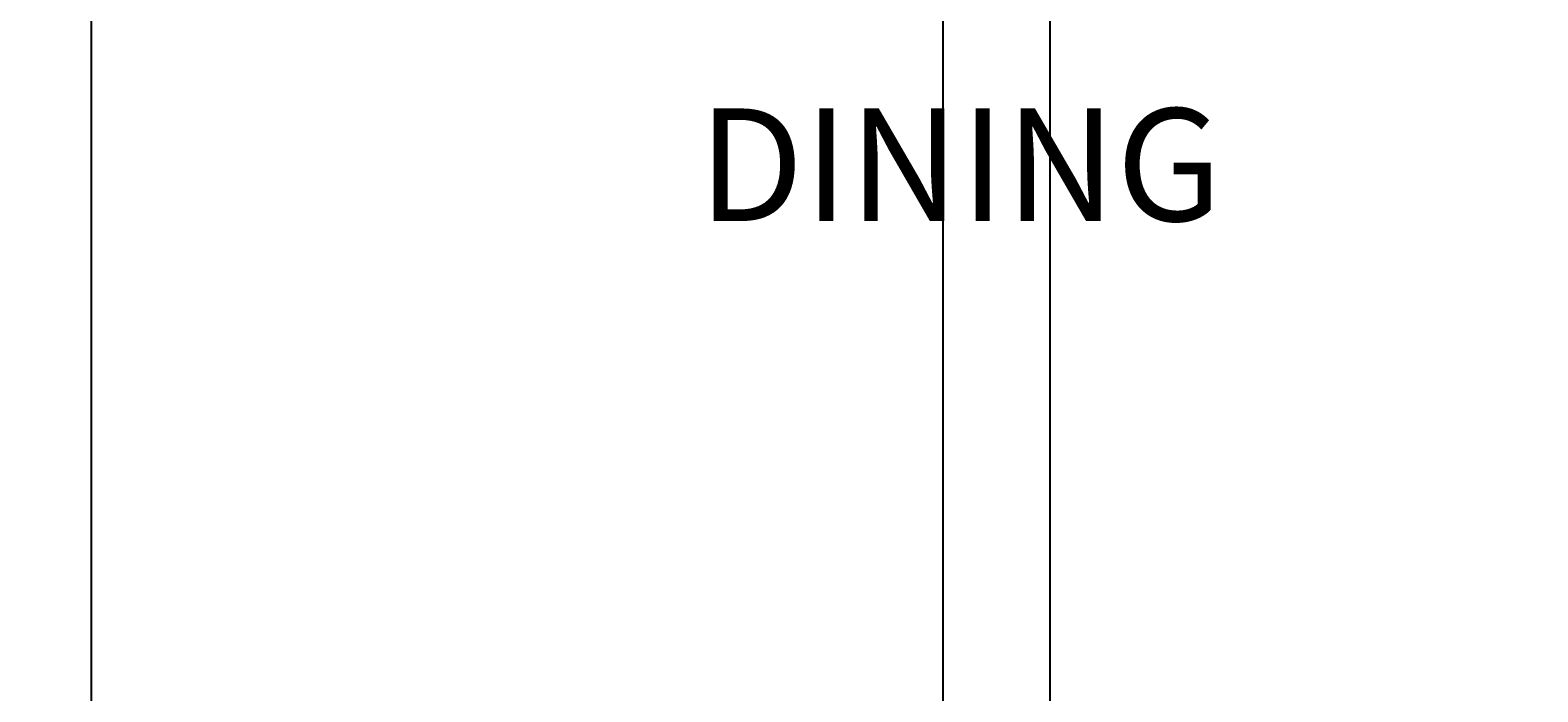
# Model space of a CAD drawing. Units: inches. Extents: x 2549 to 3108, y 1683 to 2362.
# Tile 7 of 30: x 2678 to 2762, y 1979 to 2016. Entities that reach past the tile are written whole.
import ezdxf

# ---------------------------------------------------------------- set-up
doc = ezdxf.new("R2010")
doc.units = ezdxf.units.IN
for name, color, linetype, lineweight in [('A-ANNO-DIMS', 2, 'Continuous', 18), ('A-AREA-IDEN', 7, 'Continuous', 18), ('A-FURN-PATT', 9, 'Continuous', 13)]:
    doc.layers.add(name, color=color, linetype=linetype, lineweight=lineweight)
doc.layers.add('C-PKNG-VEHI-PATT', color=251, linetype='Continuous', lineweight=13, true_color=0x636466)
doc.layers.add('C-PVMT-PATT', color=9, linetype='Continuous', lineweight=13, true_color=0xc7c8ca)
doc.styles.get("Standard").update_dxf_attribs({"font": 'arial.ttf'})
doc.dimstyles.get("Standard").update_dxf_attribs({"dimtxt": 0.18, "dimasz": 0.18, "dimexe": 0.18, "dimexo": 0.0625, "dimgap": 0.09, "dimtad": 0, "dimtih": 1, "dimtoh": 1, "dimdec": 4, "dimzin": 0, "dimdsep": 46, "dimtxsty": 'Standard', "dimcen": 0.09, "dimadec": 0, "dimazin": 0, "dimtfac": 1, "dimtdec": 4, "dimtofl": 0, "dimtmove": 0, "dimatfit": 3, "dimfxl": 1, "dimtolj": 1, "dimtzin": 0, "dimarcsym": 0})

# ---------------------------------------------------------------- blocks, each defined once
blk = doc.blocks.new('*D42')
at = {"layer": 'A-ANNO-DIMS', "color": 0, "lineweight": -2, "transparency": 16777216}
for p, q in [((2638.643, 2080.461), (2638.643, 1683.444)), ((2728.643, 2080.461), (2728.643, 1683.444)), ((2638.823, 1683.624), (2683.424, 1683.624)), ((2728.463, 1683.624), (2683.861, 1683.624))]:
    blk.add_line(p, q, dxfattribs=at)
at = {"layer": 'A-ANNO-DIMS', "color": 0, "transparency": 16777216}
for points in [[(2638.823, 1683.654), (2638.823, 1683.594), (2638.643, 1683.624)], [(2728.463, 1683.654), (2728.463, 1683.594), (2728.643, 1683.624)]]:
    blk.add_solid(points, dxfattribs=at)
at = {"layer": 'Defpoints', "color": 0, "transparency": 16777216}
for p in [(2638.643, 2080.524), (2728.643, 2080.524), (2728.643, 1683.624)]:
    blk.add_point(p, dxfattribs=at)
at = {"layer": 'A-ANNO-DIMS', "color": 0, "transparency": 16777216, "insert": (2683.643, 1683.624), "char_height": 0.18, "attachment_point": 5}
blk.add_mtext('\\A1;90', dxfattribs=at)
blk = doc.blocks.new('*D43')
at = {"layer": 'A-ANNO-DIMS', "color": 0, "lineweight": -2, "transparency": 16777216}
for p, q in [((2734.643, 2080.461), (2734.643, 1683.444)), ((2806.643, 2080.461), (2806.643, 1683.444)), ((2734.823, 1683.624), (2770.425, 1683.624)), ((2806.463, 1683.624), (2770.86, 1683.624))]:
    blk.add_line(p, q, dxfattribs=at)
at = {"layer": 'A-ANNO-DIMS', "color": 0, "transparency": 16777216}
for points in [[(2734.823, 1683.654), (2734.823, 1683.594), (2734.643, 1683.624)], [(2806.463, 1683.654), (2806.463, 1683.594), (2806.643, 1683.624)]]:
    blk.add_solid(points, dxfattribs=at)
at = {"layer": 'Defpoints', "color": 0, "transparency": 16777216}
for p in [(2734.643, 2080.524), (2806.643, 2080.524), (2806.643, 1683.624)]:
    blk.add_point(p, dxfattribs=at)
at = {"layer": 'A-ANNO-DIMS', "color": 0, "transparency": 16777216, "insert": (2770.643, 1683.624), "char_height": 0.18, "attachment_point": 5}
blk.add_mtext('\\A1;72', dxfattribs=at)
blk = doc.blocks.new('*D44')
at = {"layer": 'A-ANNO-DIMS', "color": 0, "lineweight": -2, "transparency": 16777216}
for p, q in [((2662.643, 2040.993), (2662.643, 1683.444)), ((2806.643, 2016.129), (2806.643, 1683.444)), ((2662.823, 1683.624), (2734.363, 1683.624)), ((2806.463, 1683.624), (2734.923, 1683.624))]:
    blk.add_line(p, q, dxfattribs=at)
at = {"layer": 'A-ANNO-DIMS', "color": 0, "transparency": 16777216}
for points in [[(2662.823, 1683.654), (2662.823, 1683.594), (2662.643, 1683.624)], [(2806.463, 1683.654), (2806.463, 1683.594), (2806.643, 1683.624)]]:
    blk.add_solid(points, dxfattribs=at)
at = {"layer": 'Defpoints', "color": 0, "transparency": 16777216}
for p in [(2662.643, 2041.056), (2806.643, 2016.191), (2806.643, 1683.624)]:
    blk.add_point(p, dxfattribs=at)
at = {"layer": 'A-ANNO-DIMS', "color": 0, "transparency": 16777216, "insert": (2734.643, 1683.624), "char_height": 0.18, "attachment_point": 5}
blk.add_mtext('\\A1;144', dxfattribs=at)
blk = doc.blocks.new('*D59')
at = {"layer": 'A-ANNO-DIMS', "color": 0, "lineweight": -2, "transparency": 16777216}
for p, q in [((2680.978, 1761.586), (2680.978, 2362.323)), ((2786.158, 1761.586), (2786.158, 2362.323)), ((2681.158, 2362.143), (2733.112, 2362.143)), ((2785.978, 2362.143), (2734.023, 2362.143))]:
    blk.add_line(p, q, dxfattribs=at)
at = {"layer": 'A-ANNO-DIMS', "color": 0, "transparency": 16777216}
for points in [[(2681.158, 2362.173), (2681.158, 2362.113), (2680.978, 2362.143)], [(2785.978, 2362.173), (2785.978, 2362.113), (2786.158, 2362.143)]]:
    blk.add_solid(points, dxfattribs=at)
at = {"layer": 'Defpoints', "color": 0, "transparency": 16777216}
for p in [(2786.158, 2362.143), (2680.978, 1761.524), (2786.158, 1761.524)]:
    blk.add_point(p, dxfattribs=at)
at = {"layer": 'A-ANNO-DIMS', "color": 0, "transparency": 16777216, "insert": (2733.568, 2362.143), "char_height": 0.18, "attachment_point": 5}
blk.add_mtext('\\A1;105.18', dxfattribs=at)

msp = doc.modelspace()

# ---------------------------------------------------------------- hatches: boundary and pattern name
at = {"layer": 'A-FURN-PATT', "transparency": 33554567}
h = msp.add_hatch(color=256, dxfattribs=at)
h.dxf.hatch_style = 1
h.paths.add_polyline_path([(2708.7147, 2271.6737), (2675.2813, 2271.6737), (2675.2813, 2262.0404), (2708.7147, 2262.0404)])
h.paths.add_polyline_path([(2980.8246, 2271.6737), (2947.3913, 2271.6737), (2947.3913, 2262.0404), (2980.8246, 2262.0404)])
h.paths.add_polyline_path([(2748.8496, 2101.6383), (2798.148, 2101.6383), (2798.148, 2111.4248), (2748.8496, 2111.4248)], flags=9)
h.paths.add_polyline_path([(2685.2081, 2101.489), (2719.3253, 2101.489), (2719.3253, 2111.2819), (2685.2081, 2111.2819)], flags=9)
h.paths.add_polyline_path([(2814.6852, 1907.1328), (2847.8384, 1907.1328), (2847.8384, 1916.9258), (2814.6852, 1916.9258)], flags=9)
h.paths.add_polyline_path([(2814.3906, 1835.5864), (2848.0172, 1835.5864), (2848.0172, 1845.3794), (2814.3906, 1845.3794)], flags=9)
h.paths.add_polyline_path([(2800.5245, 1759.1674), (2853.7435, 1759.1674), (2853.7435, 1768.954), (2800.5245, 1768.954)], flags=9)
h.paths.add_polyline_path([(2972.4611, 1807.3305), (3015.3943, 1807.3305), (3015.3943, 1817.117), (2972.4611, 1817.117)], flags=9)
h.paths.add_polyline_path([(2902.3327, 1888.6731), (2937.9131, 1888.6731), (2937.9131, 1898.4661), (2902.3327, 1898.4661)], flags=9)
h.paths.add_polyline_path([(2712.1779, 1878.9039), (2754.1257, 1878.9039), (2754.1257, 1888.6904), (2712.1779, 1888.6904)], flags=9)
h.paths.add_polyline_path([(2614.0056, 2012.812), (2650.0251, 2012.812), (2650.0251, 2022.4371), (2614.0056, 2022.4371)], flags=9)
h.paths.add_polyline_path([(2713.3129, 2003.1645), (2747.4237, 2003.1645), (2747.4237, 2012.951), (2713.3129, 2012.951)], flags=9)
h.paths.add_polyline_path([(2950.1379, 2001.6934), (2982.2992, 2001.6934), (2982.2992, 2011.48), (2950.1379, 2011.48)], flags=9)
h.paths.add_polyline_path([(2940.864, 2238.5537), (2997.5066, 2238.5537), (2997.5066, 2248.3466), (2940.864, 2248.3466)], flags=9)
h.paths.add_polyline_path([(2821.5457, 2202.8348), (2855.663, 2202.8348), (2855.663, 2212.6278), (2821.5457, 2212.6278)], flags=9)
h.paths.add_polyline_path([(2661.8026, 2238.6249), (2718.4451, 2238.6249), (2718.4451, 2248.4179), (2661.8026, 2248.4179)], flags=9)
h = msp.add_hatch(color=256, dxfattribs=at)
h.dxf.hatch_style = 1
h.paths.add_polyline_path([(2906.5064, 1905.2148), (2905.2584, 1904.3827), (2907.0611, 1900.7772), (2908.3092, 1901.6092)])
h.paths.add_polyline_path([(2936.522, 1914.8044), (2935.2739, 1915.6364), (2932.6391, 1912.5856), (2933.8871, 1911.7535)])
h.paths.add_polyline_path([(2950.2508, 1905.6518), (2949.0027, 1906.4839), (2947.1999, 1902.8783), (2948.448, 1902.0463)])
h.paths.add_polyline_path([(2958.5713, 1918.1326), (2956.9072, 1919.242), (2952.4696, 1908.98, 1.3874274), (2954.9657, 1907.3159)])
h.paths.add_polyline_path([(2945.2585, 1927.0078), (2943.5944, 1928.1172), (2934.9965, 1920.6287, 1.3874274), (2937.4927, 1918.9646)])
h.paths.add_polyline_path([(2748.8496, 2101.6383), (2798.148, 2101.6383), (2798.148, 2111.4248), (2748.8496, 2111.4248)], flags=9)
h.paths.add_polyline_path([(2685.2081, 2101.489), (2719.3253, 2101.489), (2719.3253, 2111.2819), (2685.2081, 2111.2819)], flags=9)
h.paths.add_polyline_path([(2814.6852, 1907.1328), (2847.8384, 1907.1328), (2847.8384, 1916.9258), (2814.6852, 1916.9258)], flags=9)
h.paths.add_polyline_path([(2814.3906, 1835.5864), (2848.0172, 1835.5864), (2848.0172, 1845.3794), (2814.3906, 1845.3794)], flags=9)
h.paths.add_polyline_path([(2800.5245, 1759.1674), (2853.7435, 1759.1674), (2853.7435, 1768.954), (2800.5245, 1768.954)], flags=9)
h.paths.add_polyline_path([(2972.4611, 1807.3305), (3015.3943, 1807.3305), (3015.3943, 1817.117), (2972.4611, 1817.117)], flags=9)
h.paths.add_polyline_path([(2902.3327, 1888.6731), (2937.9131, 1888.6731), (2937.9131, 1898.4661), (2902.3327, 1898.4661)], flags=9)
h.paths.add_polyline_path([(2712.1779, 1878.9039), (2754.1257, 1878.9039), (2754.1257, 1888.6904), (2712.1779, 1888.6904)], flags=9)
h.paths.add_polyline_path([(2614.0056, 2012.812), (2650.0251, 2012.812), (2650.0251, 2022.4371), (2614.0056, 2022.4371)], flags=9)
h.paths.add_polyline_path([(2713.3129, 2003.1645), (2747.4237, 2003.1645), (2747.4237, 2012.951), (2713.3129, 2012.951)], flags=9)
h.paths.add_polyline_path([(2950.1379, 2001.6934), (2982.2992, 2001.6934), (2982.2992, 2011.48), (2950.1379, 2011.48)], flags=9)
h.paths.add_polyline_path([(2940.864, 2238.5537), (2997.5066, 2238.5537), (2997.5066, 2248.3466), (2940.864, 2248.3466)], flags=9)
h.paths.add_polyline_path([(2821.5457, 2202.8348), (2855.663, 2202.8348), (2855.663, 2212.6278), (2821.5457, 2212.6278)], flags=9)
h.paths.add_polyline_path([(2661.8026, 2238.6249), (2718.4451, 2238.6249), (2718.4451, 2248.4179), (2661.8026, 2248.4179)], flags=9)
at = {"layer": 'C-PKNG-VEHI-PATT'}
h = msp.add_hatch(color=256, dxfattribs=at)
h.dxf.hatch_style = 1
edge = h.paths.add_edge_path()
edge.add_ellipse((2935.7258, 1791.964), major_axis=(-50.66, 0), ratio=0.8423039, start_angle=248.165046, end_angle=265.722579)
edge.add_line((2938.911, 1834.5507), (2925.8653, 1834.5507))
edge.add_ellipse((2929.0505, 1791.964), major_axis=(50.66, 0), ratio=0.8423039, start_angle=94.277421, end_angle=111.834954)
edge.add_line((2912.8508, 1832.3947), (2914.2044, 1822.2495))
edge.add_ellipse((2930.6538, 1783.1023), major_axis=(-49.3014, 0), ratio=0.8423039, start_angle=-85.12993, end_angle=-67.208085, ccw=False)
edge.add_line((2927.1247, 1824.5225), (2937.6516, 1824.5225))
edge.add_ellipse((2934.1225, 1783.1023), major_axis=(49.3014, 0), ratio=0.8423039, start_angle=67.208085, end_angle=85.12993, ccw=False)
edge.add_line((2950.5719, 1822.2495), (2951.9255, 1832.3947))
edge = h.paths.add_edge_path()
edge.add_ellipse((2903.4793, 1857.3351), major_axis=(-34.7979, 0), ratio=0.8423039, start_angle=180, end_angle=209.43857)
edge.add_ellipse((2961.297, 1857.3351), major_axis=(34.7979, 0), ratio=0.8423039, start_angle=150.56143, end_angle=180)
edge.add_line((2926.4991, 1857.3351), (2926.4991, 1843.7609))
edge.add_ellipse((2924.1251, 1844.3143), major_axis=(-0.2209, 3.9278), ratio=0.6038336, start_angle=89.002014, end_angle=253.657408, ccw=False)
edge.add_line((2921.7512, 1844.2222), (2921.7512, 1853.3975))
edge.add_line((2921.7512, 1853.3975), (2925.269, 1855.8484))
edge.add_ellipse((2925.4782, 1855.4931), major_axis=(0.4584, 0), ratio=0.8423039, start_angle=90, end_angle=134.480211, ccw=False)
edge.add_line((2925.4782, 1855.8792), (2926.4991, 1855.8792))
edge.add_line((2926.4991, 1855.8792), (2926.4991, 1857.3351))
edge.add_ellipse((2961.297, 1857.3351), major_axis=(34.7979, 0), ratio=0.8423039, start_angle=150.56143, end_angle=180, ccw=False)
edge.add_line((2932.3882, 1873.6501), (2932.3882, 1875.7801))
edge.add_ellipse((2932.3882, 1875.3939), major_axis=(0.4584, 0), ratio=0.8423039, start_angle=90, end_angle=127.93313)
edge.add_line((2932.1366, 1875.7167), (2928.5915, 1873.7564))
edge.add_ellipse((2899.9271, 2002.4692), major_axis=(155.4756, 0), ratio=0.84230387, start_angle=-80.743434, end_angle=-77.445067, ccw=False)
edge.add_ellipse((2949.4402, 1715.2151), major_axis=(-189.1422, 0), ratio=0.84230387, start_angle=-79.790461, end_angle=-77.555373)
edge.add_ellipse((3300.3614, 1852.5642), major_axis=(-386.1662, 0), ratio=0.84230387, start_angle=-2.863715, end_angle=2.198541)
edge.add_ellipse((2929.0505, 1792.5159), major_axis=(-55.6192, 0), ratio=0.8423039, start_angle=-85.917589, end_angle=-72.280047, ccw=False)
edge.add_line((2925.7129, 1839.2798), (2939.0634, 1839.2798))
edge.add_ellipse((2935.7258, 1792.5159), major_axis=(55.6192, 0), ratio=0.8423039, start_angle=72.280047, end_angle=85.917589, ccw=False)
edge.add_ellipse((2564.4149, 1852.5642), major_axis=(-386.1662, 0), ratio=0.84230387, start_angle=177.801459, end_angle=182.863715)
edge.add_ellipse((2915.3361, 1715.2151), major_axis=(189.1422, 0), ratio=0.84230387, start_angle=77.555373, end_angle=79.790461)
edge.add_ellipse((2964.8492, 2002.4692), major_axis=(-155.4756, 0), ratio=0.84230387, start_angle=77.445067, end_angle=80.743434, ccw=False)
edge.add_line((2936.1848, 1873.7564), (2932.6397, 1875.7167))
edge.add_ellipse((2932.3882, 1875.3939), major_axis=(0.4584, 0), ratio=0.8423039, start_angle=52.06687, end_angle=90)
edge.add_line((2932.3882, 1875.7801), (2932.3882, 1873.6501))
edge.add_ellipse((2903.4793, 1857.3351), major_axis=(-34.7979, 0), ratio=0.8423039, start_angle=180, end_angle=209.43857, ccw=False)
edge.add_line((2938.2772, 1857.3351), (2938.2772, 1855.8792))
edge.add_line((2938.2772, 1855.8792), (2939.4059, 1855.8792))
edge.add_ellipse((2939.2981, 1855.4931), major_axis=(-0.4584, 0), ratio=0.8423039, start_angle=225.519789, end_angle=270, ccw=False)
edge.add_line((2939.5903, 1855.7906), (2943.0251, 1853.3975))
edge.add_line((2943.0251, 1853.3975), (2943.0251, 1844.2222))
edge.add_ellipse((2940.6512, 1844.3143), major_axis=(0.2209, 3.9278), ratio=0.6038336, start_angle=106.342592, end_angle=270.997986, ccw=False)
edge.add_line((2938.2772, 1843.7609), (2938.2772, 1857.3351))
edge = h.paths.add_edge_path()
edge.add_ellipse((2932.3882, 1865.1973), major_axis=(91.081, 0), ratio=0.8423039, start_angle=256.401865, end_angle=283.598135, ccw=False)
edge.add_line((2914.2044, 1790.0239), (2914.2044, 1778.3622))
edge.add_ellipse((2932.3882, 1853.5356), major_axis=(91.081, 0), ratio=0.8423039, start_angle=256.401865, end_angle=283.598135)
edge.add_line((2950.5719, 1778.3622), (2950.5719, 1790.0239))
edge = h.paths.add_edge_path()
edge.add_ellipse((2948.7383, 1772.3145), major_axis=(1.8336, 0), ratio=0.8423039, start_angle=0, end_angle=90)
edge.add_line((2948.7383, 1773.859), (2916.038, 1773.859))
edge.add_ellipse((2916.038, 1772.3145), major_axis=(1.8336, 0), ratio=0.8423039, start_angle=90, end_angle=180)
edge.add_line((2914.2044, 1772.3145), (2914.2044, 1760.2558))
edge.add_line((2914.2044, 1760.2558), (2950.5719, 1760.2558))
edge.add_line((2950.5719, 1760.2558), (2950.5719, 1772.3145))
h.paths.add_polyline_path([(2748.8496, 2101.6383), (2798.148, 2101.6383), (2798.148, 2111.4248), (2748.8496, 2111.4248)], flags=9)
h.paths.add_polyline_path([(2685.2081, 2101.489), (2719.3253, 2101.489), (2719.3253, 2111.2819), (2685.2081, 2111.2819)], flags=9)
h.paths.add_polyline_path([(2814.6852, 1907.1328), (2847.8384, 1907.1328), (2847.8384, 1916.9258), (2814.6852, 1916.9258)], flags=9)
h.paths.add_polyline_path([(2814.3906, 1835.5864), (2848.0172, 1835.5864), (2848.0172, 1845.3794), (2814.3906, 1845.3794)], flags=9)
h.paths.add_polyline_path([(2800.5245, 1759.1674), (2853.7435, 1759.1674), (2853.7435, 1768.954), (2800.5245, 1768.954)], flags=9)
h.paths.add_polyline_path([(2972.4611, 1807.3305), (3015.3943, 1807.3305), (3015.3943, 1817.117), (2972.4611, 1817.117)], flags=9)
h.paths.add_polyline_path([(2902.3327, 1888.6731), (2937.9131, 1888.6731), (2937.9131, 1898.4661), (2902.3327, 1898.4661)], flags=9)
h.paths.add_polyline_path([(2712.1779, 1878.9039), (2754.1257, 1878.9039), (2754.1257, 1888.6904), (2712.1779, 1888.6904)], flags=9)
h.paths.add_polyline_path([(2614.0056, 2012.812), (2650.0251, 2012.812), (2650.0251, 2022.4371), (2614.0056, 2022.4371)], flags=9)
h.paths.add_polyline_path([(2713.3129, 2003.1645), (2747.4237, 2003.1645), (2747.4237, 2012.951), (2713.3129, 2012.951)], flags=9)
h.paths.add_polyline_path([(2950.1379, 2001.6934), (2982.2992, 2001.6934), (2982.2992, 2011.48), (2950.1379, 2011.48)], flags=9)
h.paths.add_polyline_path([(2940.864, 2238.5537), (2997.5066, 2238.5537), (2997.5066, 2248.3466), (2940.864, 2248.3466)], flags=9)
h.paths.add_polyline_path([(2821.5457, 2202.8348), (2855.663, 2202.8348), (2855.663, 2212.6278), (2821.5457, 2212.6278)], flags=9)
h.paths.add_polyline_path([(2661.8026, 2238.6249), (2718.4451, 2238.6249), (2718.4451, 2248.4179), (2661.8026, 2248.4179)], flags=9)
at = {"layer": 'C-PVMT-PATT'}
h = msp.add_hatch(color=256, dxfattribs=at)
h.dxf.hatch_style = 1
h.paths.add_polyline_path([(3067.6427, 2305.5237), (2605.6427, 2305.5237), (2605.6427, 2074.5237), (2629.6427, 2074.5237), (2629.6427, 2281.5237), (3043.6427, 2281.5237), (3043.6427, 1885.5237), (3043.6427, 1872.8745), (3031.1672, 1872.8745), (3031.1672, 1862.5731), (2995.8054, 1862.5731), (2995.8054, 1872.8745), (2983.1752, 1872.8745), (2983.1752, 1885.5237), (2881.6427, 1885.5237), (2881.6427, 1795.5237), (2751.0977, 1795.5237), (2751.0977, 1761.5237), (2786.1577, 1761.5237), (2786.1577, 1723.5237), (2881.84, 1723.5237), (2881.84, 1714.5237), (3067.6427, 1714.5237), (3067.6427, 1723.5237)])
edge = h.paths.add_edge_path(flags=16)
edge.add_ellipse((2949.4402, 1710.9683), major_axis=(-194.1014, 0), ratio=0.84230387, start_angle=-77.874034, end_angle=-76.219471, ccw=False)
edge.add_ellipse((2949.4402, 1715.2151), major_axis=(-189.1422, 0), ratio=0.84230387, start_angle=-79.790461, end_angle=-77.555373, ccw=False)
edge.add_ellipse((2899.9271, 2002.4692), major_axis=(155.4756, 0), ratio=0.84230387, start_angle=-80.743434, end_angle=-77.445067)
edge.add_line((2928.5915, 1873.7564), (2932.3882, 1875.8558))
edge.add_line((2932.3882, 1875.8558), (2936.1848, 1873.7564))
edge.add_ellipse((2964.8492, 2002.4692), major_axis=(-155.4756, 0), ratio=0.84230387, start_angle=77.445067, end_angle=80.743434)
edge.add_ellipse((2915.3361, 1715.2151), major_axis=(189.1422, 0), ratio=0.84230387, start_angle=77.555373, end_angle=79.790461, ccw=False)
edge.add_ellipse((2915.3361, 1710.9683), major_axis=(-194.1014, 0), ratio=0.84230387, start_angle=256.219471, end_angle=257.874034, ccw=False)
edge.add_ellipse((2628.2871, 1850.2612), major_axis=(-327.2532, 0), ratio=0.84230387, start_angle=182.17995, end_angle=183.650428, ccw=False)
edge.add_ellipse((2955.5637, 1861.9334), major_axis=(-0.9168, 0), ratio=0.8423039, start_angle=180, end_angle=270, ccw=False)
edge.add_line((2956.4805, 1862.3857), (2956.4805, 1846.4866))
edge.add_ellipse((2955.5637, 1846.939), major_axis=(-0.9168, 0), ratio=0.8423039, start_angle=90, end_angle=180, ccw=False)
edge.add_ellipse((-3607.0606, 1835.832), major_axis=(-6562.6242, 0), ratio=0.84230387, start_angle=179.61613322, end_angle=180.09022909, ccw=False)
edge.add_ellipse((2955.5637, 1791.0926), major_axis=(0.9168, 0), ratio=0.8423039, start_angle=0, end_angle=90, ccw=False)
edge.add_line((2956.4805, 1791.545), (2956.4805, 1775.6459))
edge.add_ellipse((2955.5637, 1776.0982), major_axis=(0.9168, 0), ratio=0.8423039, start_angle=270, end_angle=360, ccw=False)
edge.add_ellipse((-3607.0606, 1835.832), major_axis=(-6562.6242, 0), ratio=0.84230387, start_angle=179.3813568, end_angle=179.47172853, ccw=False)
edge.add_ellipse((2954.5907, 1763.8768), major_axis=(-1.3752, 0), ratio=0.8423039, start_angle=179.371763, end_angle=248.464757, ccw=False)
edge.add_ellipse((-3607.519, 1835.832), major_axis=(-6564.0409, 0), ratio=0.842303863, start_angle=179.35344594, end_angle=179.37176282, ccw=False)
edge.add_ellipse((2952.6829, 1761.8002), major_axis=(3.2503, 0), ratio=0.8423039, start_angle=-90, end_angle=-0.646554, ccw=False)
edge.add_line((2952.6829, 1759.0625), (2912.0934, 1759.0625))
edge.add_ellipse((2912.0934, 1761.8002), major_axis=(3.2503, 0), ratio=0.8423039, start_angle=180.646554, end_angle=270, ccw=False)
edge.add_ellipse((9472.2953, 1835.832), major_axis=(-6564.0409, 0), ratio=0.842303871, start_angle=0.62823722, end_angle=0.6465541, ccw=False)
edge.add_ellipse((2910.1856, 1763.8768), major_axis=(1.3752, 0), ratio=0.8423039, start_angle=111.535244, end_angle=180.628237, ccw=False)
edge.add_ellipse((9471.8369, 1835.832), major_axis=(-6562.6242, 0), ratio=0.84230387, start_angle=0.52827147, end_angle=0.6465541, ccw=False)
edge.add_ellipse((2909.2126, 1776.0982), major_axis=(-0.9168, 0), ratio=0.8423039, start_angle=0, end_angle=90, ccw=False)
edge.add_line((2908.2958, 1775.6459), (2908.2958, 1791.545))
edge.add_ellipse((2909.2126, 1791.0926), major_axis=(-0.9168, 0), ratio=0.8423039, start_angle=-90, end_angle=0, ccw=False)
edge.add_ellipse((9471.8369, 1835.832), major_axis=(-6562.6242, 0), ratio=0.84230387, start_angle=-0.09022909, end_angle=0.38386678, ccw=False)
edge.add_ellipse((2909.2126, 1846.939), major_axis=(-0.9168, 0), ratio=0.8423039, start_angle=0, end_angle=90, ccw=False)
edge.add_line((2908.2958, 1846.4866), (2908.2958, 1862.3857))
edge.add_ellipse((2909.2126, 1861.9334), major_axis=(0.9168, 0), ratio=0.8423039, start_angle=90, end_angle=180, ccw=False)
edge.add_ellipse((3236.4892, 1850.2612), major_axis=(327.2532, 0), ratio=0.84230387, start_angle=176.349572, end_angle=177.82005, ccw=False)
edge = h.paths.add_edge_path(flags=0)
edge.add_ellipse((2903.4793, 1857.3351), major_axis=(-34.7979, 0), ratio=0.8423039, start_angle=180, end_angle=209.43857, ccw=False)
edge.add_line((2938.2772, 1857.3351), (2938.2772, 1855.8792))
edge.add_line((2938.2772, 1855.8792), (2939.4631, 1855.8792))
edge.add_line((2939.4631, 1855.8792), (2943.0251, 1853.3975))
edge.add_line((2943.0251, 1853.3975), (2943.0251, 1844.2222))
edge.add_ellipse((2940.6512, 1844.3143), major_axis=(0.2209, 3.9278), ratio=0.6038336, start_angle=106.342592, end_angle=270.997986, ccw=False)
edge.add_line((2938.2772, 1843.7609), (2938.2772, 1857.3351))
edge.add_ellipse((2903.4793, 1857.3351), major_axis=(-34.7979, 0), ratio=0.8423039, start_angle=180, end_angle=209.43857)
edge.add_ellipse((2961.297, 1857.3351), major_axis=(34.7979, 0), ratio=0.8423039, start_angle=150.56143, end_angle=180)
edge.add_line((2926.4991, 1857.3351), (2926.4991, 1843.7609))
edge.add_ellipse((2924.1251, 1844.3143), major_axis=(-0.2209, 3.9278), ratio=0.6038336, start_angle=89.002014, end_angle=253.657408, ccw=False)
edge.add_line((2921.7512, 1844.2222), (2921.7512, 1853.3975))
edge.add_line((2921.7512, 1853.3975), (2925.3132, 1855.8792))
edge.add_line((2925.3132, 1855.8792), (2926.4991, 1855.8792))
edge.add_line((2926.4991, 1855.8792), (2926.4991, 1857.3351))
edge.add_ellipse((2961.297, 1857.3351), major_axis=(34.7979, 0), ratio=0.8423039, start_angle=150.56143, end_angle=180, ccw=False)
edge = h.paths.add_edge_path(flags=0)
edge.add_ellipse((2929.0505, 1791.964), major_axis=(50.66, 0), ratio=0.8423039, start_angle=94.277421, end_angle=111.834954, ccw=False)
edge.add_line((2925.8653, 1834.5507), (2938.911, 1834.5507))
edge.add_ellipse((2935.7258, 1791.964), major_axis=(-50.66, 0), ratio=0.8423039, start_angle=248.165046, end_angle=265.722579, ccw=False)
edge.add_line((2951.9255, 1832.3947), (2950.5719, 1822.2495))
edge.add_ellipse((2934.1225, 1783.1023), major_axis=(49.3014, 0), ratio=0.8423039, start_angle=67.208085, end_angle=85.12993)
edge.add_line((2937.6516, 1824.5225), (2927.1247, 1824.5225))
edge.add_ellipse((2930.6538, 1783.1023), major_axis=(-49.3014, 0), ratio=0.8423039, start_angle=-85.12993, end_angle=-67.208085)
edge.add_line((2914.2044, 1822.2495), (2912.8508, 1832.3947))
edge = h.paths.add_edge_path(flags=0)
edge.add_line((2910.1338, 1829.4651), (2912.6432, 1821.2711))
edge.add_ellipse((5203.7787, 1816.4367), major_axis=(-2291.1426, 0), ratio=0.84230387, start_angle=-0.1208974, end_angle=0.3640763)
edge.add_line((2912.7012, 1801.8782), (2910.3305, 1792.5698))
edge.add_ellipse((9471.8369, 1835.832), major_axis=(-6561.7074, 0), ratio=0.84230387, start_angle=0.05559431, end_angle=0.37776419, ccw=False)
edge = h.paths.add_edge_path(flags=0)
edge.add_ellipse((-3607.0606, 1835.832), major_axis=(6561.7074, 0), ratio=0.84230387, start_angle=-0.37776419, end_angle=-0.05559431, ccw=False)
edge.add_line((2954.4458, 1792.5698), (2952.0751, 1801.8782))
edge.add_ellipse((660.9976, 1816.4367), major_axis=(2291.1426, 0), ratio=0.84230387, start_angle=-0.3640763, end_angle=0.1208974)
edge.add_line((2952.1331, 1821.2711), (2954.6425, 1829.4651))
edge = h.paths.add_edge_path(flags=0)
edge.add_ellipse((2932.3882, 1865.1973), major_axis=(91.081, 0), ratio=0.8423039, start_angle=256.401865, end_angle=283.598135)
edge.add_line((2950.5719, 1790.0239), (2950.5719, 1778.3622))
edge.add_ellipse((2932.3882, 1853.5356), major_axis=(91.081, 0), ratio=0.8423039, start_angle=256.401865, end_angle=283.598135, ccw=False)
edge.add_line((2914.2044, 1778.3622), (2914.2044, 1790.0239))
edge = h.paths.add_edge_path(flags=0)
edge.add_line((2916.038, 1773.859), (2948.7383, 1773.859))
edge.add_ellipse((2948.7383, 1772.3145), major_axis=(1.8336, 0), ratio=0.8423039, start_angle=0, end_angle=90, ccw=False)
edge.add_line((2950.5719, 1772.3145), (2950.5719, 1760.2558))
edge.add_line((2950.5719, 1760.2558), (2914.2044, 1760.2558))
edge.add_line((2914.2044, 1760.2558), (2914.2044, 1772.3145))
edge.add_ellipse((2916.038, 1772.3145), major_axis=(1.8336, 0), ratio=0.8423039, start_angle=90, end_angle=180, ccw=False)
h.paths.add_polyline_path([(2629.6427, 1978.5237), (2605.6427, 1978.5237), (2605.6427, 1723.5237), (2629.6427, 1723.5237), (2629.6427, 1795.5237)], flags=17)
h.paths.add_polyline_path([(2800.5245, 1759.1674), (2853.7435, 1759.1674), (2853.7435, 1768.954), (2800.5245, 1768.954)], flags=24)
h.paths.add_polyline_path([(2972.4611, 1807.3305), (3015.3943, 1807.3305), (3015.3943, 1817.117), (2972.4611, 1817.117)], flags=24)

# ---------------------------------------------------------------- texts
at = {"layer": 'A-AREA-IDEN'}
msp.add_text('DINING', height=6.30916, dxfattribs=at).set_placement((2714.944, 2004.9032))

# ---------------------------------------------------------------- dimensions: what is measured, and where the dimension line sits
at = {"layer": 'A-ANNO-DIMS'}
for base, p1, p2, override, picture, middle in [((2786.1577, 2362.1425), (2680.9778, 1761.5237), (2786.1577, 1761.5237), {"dimdec": 2, "dimlfac": 1, "dimrnd": 0, "dimzin": 0, "dimdsep": 46, "dimlunit": 2}, '*D59', (2733.5678, 2362.1425)), ((2728.6427, 1683.6237), (2638.6427, 2080.5237), (2728.6427, 2080.5237), {"dimdec": 0, "dimlfac": 1, "dimrnd": 0, "dimzin": 0, "dimdsep": 46, "dimlunit": 2}, '*D42', (2683.6427, 1683.6237)), ((2806.6427, 1683.6237), (2734.6427, 2080.5237), (2806.6427, 2080.5237), {"dimdec": 0, "dimlfac": 1, "dimrnd": 0, "dimzin": 0, "dimdsep": 46, "dimlunit": 2}, '*D43', (2770.6427, 1683.6237)), ((2806.6427, 1683.6237), (2662.6427, 2041.0557), (2806.6427, 2016.1911), {"dimdec": 0, "dimlfac": 1, "dimrnd": 0, "dimzin": 0, "dimdsep": 46, "dimlunit": 2}, '*D44', (2734.6427, 1683.6237))]:
    dim = msp.add_linear_dim(base=base, p1=p1, p2=p2, dimstyle='Standard', override=override, dxfattribs=at)
    dim.commit()
    dim.dimension.update_dxf_attribs({"geometry": picture, "text_midpoint": middle})

doc.saveas('drawing.dxf')
